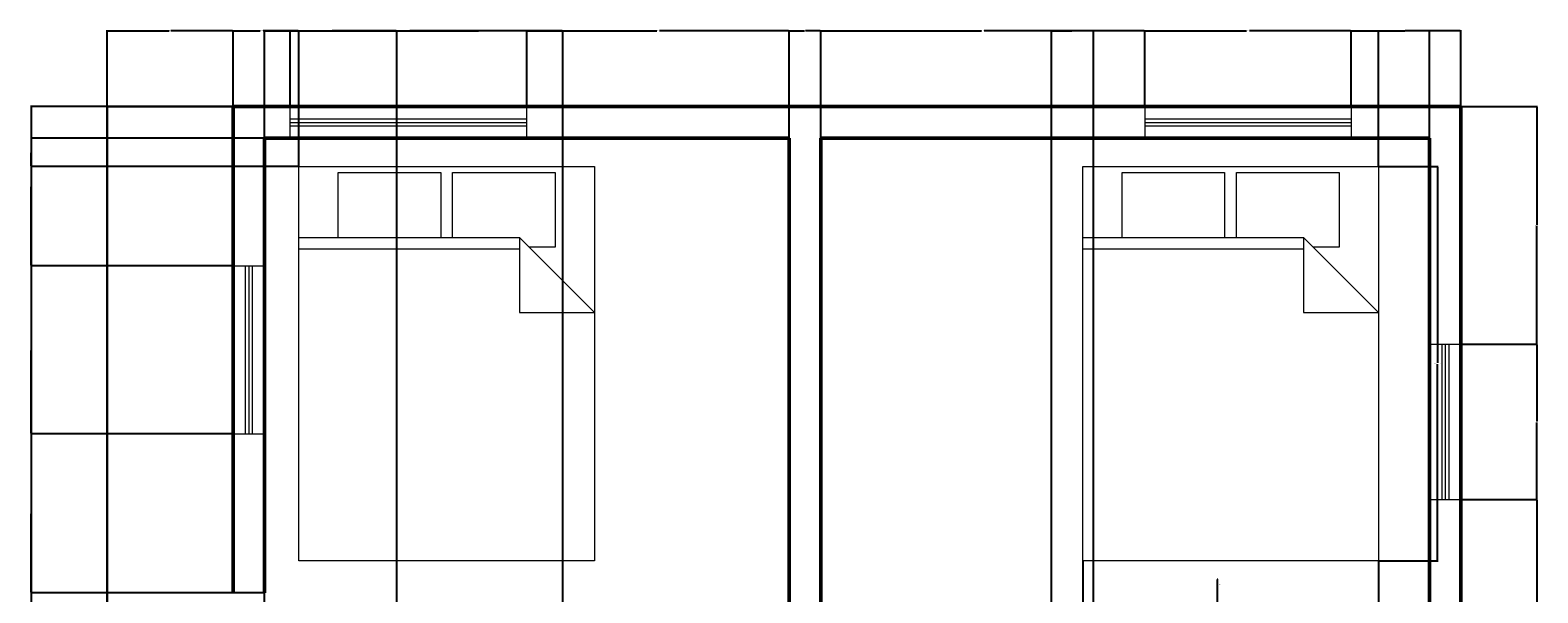
# Model space of a CAD drawing. Units: feet. Extents: x 2387 to 2818, y 1569 to 2046.
# Tile 4 of 4: x 2387 to 2818, y 1885 to 2046. Entities that reach past the tile are written whole.
import ezdxf

# ---------------------------------------------------------------- set-up
doc = ezdxf.new("R2010")
doc.units = ezdxf.units.FT
for name, color, linetype, lineweight in [('A-ANNO-DIMS', 2, 'Continuous', 18), ('A-DOOR', 3, 'Continuous', 25), ('A-FLOR-BALC', 7, 'Continuous', 30), ('A-FURN', 8, 'Continuous', 18), ('A-GLAZ', 4, 'Continuous', 18), ('A-WALL', 7, 'Continuous', 50)]:
    doc.layers.add(name, color=color, linetype=linetype, lineweight=lineweight)
doc.styles.get("Standard").update_dxf_attribs({"font": 'arial.ttf'})
doc.dimstyles.get("Standard").update_dxf_attribs({"dimtxt": 0.18, "dimasz": 0.18, "dimexe": 0.18, "dimexo": 0.0625, "dimgap": 0.09, "dimtad": 0, "dimtih": 1, "dimtoh": 1, "dimdec": 4, "dimzin": 0, "dimdsep": 46, "dimtxsty": 'Standard', "dimcen": 0.09, "dimadec": 0, "dimazin": 0, "dimtfac": 1, "dimtdec": 4, "dimtofl": 0, "dimtmove": 0, "dimatfit": 3, "dimfxl": 1, "dimtolj": 1, "dimtzin": 0, "dimarcsym": 0})

# ---------------------------------------------------------------- blocks, each defined once
blk = doc.blocks.new('Bed - Queen')
for p, q in [((0, -80.00003), (0, 0)), ((0, 0), (59.99999, 0)), ((59.99999, 0), (59.99999, -80.00003)), ((7.99999, -1.2), (28.79998, -1.2)), ((7.99999, -14.4), (7.99999, -1.2)), ((28.79998, -1.2), (28.79998, -14.4)), ((31.19999, -1.2), (51.99999, -1.2)), ((31.19999, -14.4), (31.19999, -1.2)), ((51.99999, -1.2), (51.99999, -16.4)), ((0, -14.4), (44.8, -14.4)), ((59.99999, -29.6), (44.8, -14.4)), ((44.8, -14.4), (44.8, -29.6)), ((44.8, -16.8), (0, -16.8)), ((51.99999, -16.4), (46.79936, -16.4)), ((44.8, -29.6), (59.99999, -29.6)), ((59.99999, -80.00003), (0, -80.00003))]:
    blk.add_line(p, q)
blk = doc.blocks.new('*D11')
at = {"layer": 'A-ANNO-DIMS', "color": 0, "lineweight": -2, "transparency": 16777216}
for p, q in [((2772.22, 2006.71), (2789.25, 2006.71)), ((2789.07, 2006.53), (2789.07, 1950.54)), ((2789.07, 1894.17), (2789.07, 1950.16)), ((2772.22, 1893.99), (2789.25, 1893.99))]:
    blk.add_line(p, q, dxfattribs=at)
at = {"layer": 'A-ANNO-DIMS', "color": 0, "transparency": 16777216}
for points in [[(2789.04, 2006.53), (2789.1, 2006.53), (2789.07, 2006.71)], [(2789.04, 1894.17), (2789.1, 1894.17), (2789.07, 1893.99)]]:
    blk.add_solid(points, dxfattribs=at)
at = {"layer": 'Defpoints', "color": 0, "transparency": 16777216}
for p in [(2772.16, 2006.71), (2789.07, 2006.71), (2772.16, 1893.99)]:
    blk.add_point(p, dxfattribs=at)
at = {"layer": 'A-ANNO-DIMS', "color": 0, "transparency": 16777216, "insert": (2789.07, 1950.35), "char_height": 0.18, "attachment_point": 5}
blk.add_mtext('\\A1;QUEEN BED 113 TYP.', dxfattribs=at)
blk = doc.blocks.new('*D12')
at = {"layer": 'A-ANNO-DIMS', "color": 0, "lineweight": -2, "transparency": 16777216}
for p, q in [((2687.62, 1893.93), (2687.62, 1876.9)), ((2772.16, 1893.93), (2772.16, 1876.9)), ((2687.8, 1877.08), (2729.36, 1877.08)), ((2771.98, 1877.08), (2730.42, 1877.08))]:
    blk.add_line(p, q, dxfattribs=at)
at = {"layer": 'A-ANNO-DIMS', "color": 0, "transparency": 16777216}
for points in [[(2687.8, 1877.11), (2687.8, 1877.05), (2687.62, 1877.08)], [(2771.98, 1877.11), (2771.98, 1877.05), (2772.16, 1877.08)]]:
    blk.add_solid(points, dxfattribs=at)
at = {"layer": 'Defpoints', "color": 0, "transparency": 16777216}
for p in [(2687.62, 1893.99), (2772.16, 1893.99), (2772.16, 1877.08)]:
    blk.add_point(p, dxfattribs=at)
at = {"layer": 'A-ANNO-DIMS', "color": 0, "transparency": 16777216, "insert": (2729.89, 1877.08), "char_height": 0.18, "attachment_point": 5}
blk.add_mtext('\\A1;85 TYP.', dxfattribs=at)
blk = doc.blocks.new('*D28')
at = {"layer": 'A-ANNO-DIMS', "color": 0, "lineweight": -2, "transparency": 16777216}
for p, q in [((2408.67, 2023.82), (2386.88, 2023.82)), ((2387.06, 2023.64), (2387.06, 1807.51)), ((2387.06, 1591), (2387.06, 1807.14)), ((2408.67, 1590.82), (2386.88, 1590.82))]:
    blk.add_line(p, q, dxfattribs=at)
at = {"layer": 'A-ANNO-DIMS', "color": 0, "transparency": 16777216}
for points in [[(2387.03, 2023.64), (2387.09, 2023.64), (2387.06, 2023.82)], [(2387.03, 1591), (2387.09, 1591), (2387.06, 1590.82)]]:
    blk.add_solid(points, dxfattribs=at)
at = {"layer": 'Defpoints', "color": 0, "transparency": 16777216}
for p in [(2387.06, 2023.82), (2408.74, 2023.82), (2408.74, 1590.82)]:
    blk.add_point(p, dxfattribs=at)
at = {"layer": 'A-ANNO-DIMS', "color": 0, "transparency": 16777216, "insert": (2387.06, 1807.32), "char_height": 0.18, "attachment_point": 5}
blk.add_mtext('\\A1;433', dxfattribs=at)
blk = doc.blocks.new('*D29')
at = {"layer": 'A-ANNO-DIMS', "color": 0, "lineweight": -2, "transparency": 16777216}
for p, q in [((2408.74, 2023.89), (2408.74, 2045.68)), ((2408.92, 2045.5), (2426.52, 2045.5)), ((2444.56, 2045.5), (2426.95, 2045.5)), ((2444.74, 2023.89), (2444.74, 2045.68))]:
    blk.add_line(p, q, dxfattribs=at)
at = {"layer": 'A-ANNO-DIMS', "color": 0, "transparency": 16777216}
for points in [[(2408.92, 2045.53), (2408.92, 2045.47), (2408.74, 2045.5)], [(2444.56, 2045.53), (2444.56, 2045.47), (2444.74, 2045.5)]]:
    blk.add_solid(points, dxfattribs=at)
at = {"layer": 'Defpoints', "color": 0, "transparency": 16777216}
for p in [(2444.74, 2045.5), (2408.74, 2023.82), (2444.74, 2023.82)]:
    blk.add_point(p, dxfattribs=at)
at = {"layer": 'A-ANNO-DIMS', "color": 0, "transparency": 16777216, "insert": (2426.74, 2045.5), "char_height": 0.18, "attachment_point": 5}
blk.add_mtext('\\A1;36', dxfattribs=at)
blk = doc.blocks.new('*D30')
at = {"layer": 'A-ANNO-DIMS', "color": 0, "lineweight": -2, "transparency": 16777216}
for p, q in [((2444.74, 2023.89), (2444.74, 2045.68)), ((2444.92, 2045.5), (2452.46, 2045.5)), ((2460.91, 2045.5), (2453.37, 2045.5)), ((2461.09, 2023.89), (2461.09, 2045.68))]:
    blk.add_line(p, q, dxfattribs=at)
at = {"layer": 'A-ANNO-DIMS', "color": 0, "transparency": 16777216}
for points in [[(2444.92, 2045.53), (2444.92, 2045.47), (2444.74, 2045.5)], [(2460.91, 2045.53), (2460.91, 2045.47), (2461.09, 2045.5)]]:
    blk.add_solid(points, dxfattribs=at)
at = {"layer": 'Defpoints', "color": 0, "transparency": 16777216}
for p in [(2461.09, 2045.5), (2444.74, 2023.82), (2461.09, 2023.82)]:
    blk.add_point(p, dxfattribs=at)
at = {"layer": 'A-ANNO-DIMS', "color": 0, "transparency": 16777216, "insert": (2452.91, 2045.5), "char_height": 0.18, "attachment_point": 5}
blk.add_mtext('\\A1;16.356', dxfattribs=at)
blk = doc.blocks.new('*D31')
at = {"layer": 'A-ANNO-DIMS', "color": 0, "lineweight": -2, "transparency": 16777216}
for p, q in [((2461.09, 2023.89), (2461.09, 2045.68)), ((2461.27, 2045.5), (2494.51, 2045.5)), ((2528.54, 2045.5), (2495.3, 2045.5)), ((2528.72, 2023.89), (2528.72, 2045.68))]:
    blk.add_line(p, q, dxfattribs=at)
at = {"layer": 'A-ANNO-DIMS', "color": 0, "transparency": 16777216}
for points in [[(2461.27, 2045.53), (2461.27, 2045.47), (2461.09, 2045.5)], [(2528.54, 2045.53), (2528.54, 2045.47), (2528.72, 2045.5)]]:
    blk.add_solid(points, dxfattribs=at)
at = {"layer": 'Defpoints', "color": 0, "transparency": 16777216}
for p in [(2528.72, 2045.5), (2461.09, 2023.82), (2528.72, 2023.82)]:
    blk.add_point(p, dxfattribs=at)
at = {"layer": 'A-ANNO-DIMS', "color": 0, "transparency": 16777216, "insert": (2494.91, 2045.5), "char_height": 0.18, "attachment_point": 5}
blk.add_mtext('\\A1;67.63', dxfattribs=at)
blk = doc.blocks.new('*D32')
at = {"layer": 'A-ANNO-DIMS', "color": 0, "lineweight": -2, "transparency": 16777216}
for p, q in [((2528.72, 2023.89), (2528.72, 2045.68)), ((2528.9, 2045.5), (2565.84, 2045.5)), ((2603.56, 2045.5), (2566.62, 2045.5)), ((2603.74, 2014.89), (2603.74, 2045.68))]:
    blk.add_line(p, q, dxfattribs=at)
at = {"layer": 'A-ANNO-DIMS', "color": 0, "transparency": 16777216}
for points in [[(2528.9, 2045.53), (2528.9, 2045.47), (2528.72, 2045.5)], [(2603.56, 2045.53), (2603.56, 2045.47), (2603.74, 2045.5)]]:
    blk.add_solid(points, dxfattribs=at)
at = {"layer": 'Defpoints', "color": 0, "transparency": 16777216}
for p in [(2603.74, 2045.5), (2528.72, 2023.82), (2603.74, 2014.82)]:
    blk.add_point(p, dxfattribs=at)
at = {"layer": 'A-ANNO-DIMS', "color": 0, "transparency": 16777216, "insert": (2566.23, 2045.5), "char_height": 0.18, "attachment_point": 5}
blk.add_mtext('\\A1;75.02', dxfattribs=at)
blk = doc.blocks.new('*D33')
at = {"layer": 'A-ANNO-DIMS', "color": 0, "lineweight": -2, "transparency": 16777216}
for p, q in [((2603.74, 2014.89), (2603.74, 2045.68)), ((2603.92, 2045.5), (2608.09, 2045.5)), ((2612.56, 2045.5), (2608.39, 2045.5)), ((2612.74, 2014.89), (2612.74, 2045.68))]:
    blk.add_line(p, q, dxfattribs=at)
at = {"layer": 'A-ANNO-DIMS', "color": 0, "transparency": 16777216}
for points in [[(2603.92, 2045.53), (2603.92, 2045.47), (2603.74, 2045.5)], [(2612.56, 2045.53), (2612.56, 2045.47), (2612.74, 2045.5)]]:
    blk.add_solid(points, dxfattribs=at)
at = {"layer": 'Defpoints', "color": 0, "transparency": 16777216}
for p in [(2612.74, 2045.5), (2603.74, 2014.82), (2612.74, 2014.82)]:
    blk.add_point(p, dxfattribs=at)
at = {"layer": 'A-ANNO-DIMS', "color": 0, "transparency": 16777216, "insert": (2608.24, 2045.5), "char_height": 0.18, "attachment_point": 5}
blk.add_mtext('\\A1;9', dxfattribs=at)
blk = doc.blocks.new('*D34')
at = {"layer": 'A-ANNO-DIMS', "color": 0, "lineweight": -2, "transparency": 16777216}
for p, q in [((2612.74, 2014.89), (2612.74, 2045.68)), ((2612.92, 2045.5), (2658.66, 2045.5)), ((2705.18, 2045.5), (2659.44, 2045.5)), ((2705.36, 2023.89), (2705.36, 2045.68))]:
    blk.add_line(p, q, dxfattribs=at)
at = {"layer": 'A-ANNO-DIMS', "color": 0, "transparency": 16777216}
for points in [[(2612.92, 2045.53), (2612.92, 2045.47), (2612.74, 2045.5)], [(2705.18, 2045.53), (2705.18, 2045.47), (2705.36, 2045.5)]]:
    blk.add_solid(points, dxfattribs=at)
at = {"layer": 'Defpoints', "color": 0, "transparency": 16777216}
for p in [(2705.36, 2045.5), (2705.36, 2023.82), (2612.74, 2014.82)]:
    blk.add_point(p, dxfattribs=at)
at = {"layer": 'A-ANNO-DIMS', "color": 0, "transparency": 16777216, "insert": (2659.05, 2045.5), "char_height": 0.18, "attachment_point": 5}
blk.add_mtext('\\A1;92.63', dxfattribs=at)
blk = doc.blocks.new('*D35')
at = {"layer": 'A-ANNO-DIMS', "color": 0, "lineweight": -2, "transparency": 16777216}
for p, q in [((2705.36, 2023.89), (2705.36, 2045.68)), ((2705.54, 2045.5), (2734.48, 2045.5)), ((2764.21, 2045.5), (2735.27, 2045.5)), ((2764.39, 2023.89), (2764.39, 2045.68))]:
    blk.add_line(p, q, dxfattribs=at)
at = {"layer": 'A-ANNO-DIMS', "color": 0, "transparency": 16777216}
for points in [[(2705.54, 2045.53), (2705.54, 2045.47), (2705.36, 2045.5)], [(2764.21, 2045.53), (2764.21, 2045.47), (2764.39, 2045.5)]]:
    blk.add_solid(points, dxfattribs=at)
at = {"layer": 'Defpoints', "color": 0, "transparency": 16777216}
for p in [(2764.39, 2045.5), (2705.36, 2023.82), (2764.39, 2023.82)]:
    blk.add_point(p, dxfattribs=at)
at = {"layer": 'A-ANNO-DIMS', "color": 0, "transparency": 16777216, "insert": (2734.88, 2045.5), "char_height": 0.18, "attachment_point": 5}
blk.add_mtext('\\A1;59.03', dxfattribs=at)
blk = doc.blocks.new('*D36')
at = {"layer": 'A-ANNO-DIMS', "color": 0, "lineweight": -2, "transparency": 16777216}
for p, q in [((2764.39, 2023.89), (2764.39, 2045.68)), ((2764.57, 2045.5), (2779.67, 2045.5)), ((2795.56, 2045.5), (2780.46, 2045.5)), ((2795.74, 2023.89), (2795.74, 2045.68))]:
    blk.add_line(p, q, dxfattribs=at)
at = {"layer": 'A-ANNO-DIMS', "color": 0, "transparency": 16777216}
for points in [[(2764.57, 2045.53), (2764.57, 2045.47), (2764.39, 2045.5)], [(2795.56, 2045.53), (2795.56, 2045.47), (2795.74, 2045.5)]]:
    blk.add_solid(points, dxfattribs=at)
at = {"layer": 'Defpoints', "color": 0, "transparency": 16777216}
for p in [(2795.74, 2045.5), (2764.39, 2023.82), (2795.74, 2023.82)]:
    blk.add_point(p, dxfattribs=at)
at = {"layer": 'A-ANNO-DIMS', "color": 0, "transparency": 16777216, "insert": (2780.07, 2045.5), "char_height": 0.18, "attachment_point": 5}
blk.add_mtext('\\A1;31.34', dxfattribs=at)
blk = doc.blocks.new('*D37')
at = {"layer": 'A-ANNO-DIMS', "color": 0, "lineweight": -2, "transparency": 16777216}
for p, q in [((2491.59, 1599.89), (2491.59, 2045.68)), ((2491.77, 2045.5), (2514.91, 2045.5)), ((2538.86, 2045.5), (2515.71, 2045.5)), ((2539.04, 1599.89), (2539.04, 2045.68))]:
    blk.add_line(p, q, dxfattribs=at)
at = {"layer": 'A-ANNO-DIMS', "color": 0, "transparency": 16777216}
for points in [[(2491.77, 2045.53), (2491.77, 2045.47), (2491.59, 2045.5)], [(2538.86, 2045.53), (2538.86, 2045.47), (2539.04, 2045.5)]]:
    blk.add_solid(points, dxfattribs=at)
at = {"layer": 'Defpoints', "color": 0, "transparency": 16777216}
for p in [(2539.04, 2045.5), (2491.59, 1599.82), (2539.04, 1599.82)]:
    blk.add_point(p, dxfattribs=at)
at = {"layer": 'A-ANNO-DIMS', "color": 0, "transparency": 16777216, "insert": (2515.31, 2045.5), "char_height": 0.18, "attachment_point": 5}
blk.add_mtext('\\A1;47.45', dxfattribs=at)
blk = doc.blocks.new('*D38')
at = {"layer": 'A-ANNO-DIMS', "color": 0, "lineweight": -2, "transparency": 16777216}
for p, q in [((2453.74, 1599.89), (2453.74, 2045.68)), ((2453.92, 2045.5), (2472.27, 2045.5)), ((2491.41, 2045.5), (2473.06, 2045.5)), ((2491.59, 1599.89), (2491.59, 2045.68))]:
    blk.add_line(p, q, dxfattribs=at)
at = {"layer": 'A-ANNO-DIMS', "color": 0, "transparency": 16777216}
for points in [[(2453.92, 2045.53), (2453.92, 2045.47), (2453.74, 2045.5)], [(2491.41, 2045.53), (2491.41, 2045.47), (2491.59, 2045.5)]]:
    blk.add_solid(points, dxfattribs=at)
at = {"layer": 'Defpoints', "color": 0, "transparency": 16777216}
for p in [(2491.59, 2045.5), (2453.74, 1599.82), (2491.59, 1599.82)]:
    blk.add_point(p, dxfattribs=at)
at = {"layer": 'A-ANNO-DIMS', "color": 0, "transparency": 16777216, "insert": (2472.66, 2045.5), "char_height": 0.18, "attachment_point": 5}
blk.add_mtext('\\A1;37.85', dxfattribs=at)
blk = doc.blocks.new('*D47')
at = {"layer": 'A-ANNO-DIMS', "color": 0, "lineweight": -2, "transparency": 16777216}
for p, q in [((2444.67, 1930.32), (2386.88, 1930.32)), ((2387.06, 1930.14), (2387.06, 1907.76)), ((2387.06, 1885), (2387.06, 1907.39)), ((2444.67, 1884.82), (2386.88, 1884.82))]:
    blk.add_line(p, q, dxfattribs=at)
at = {"layer": 'A-ANNO-DIMS', "color": 0, "transparency": 16777216}
for points in [[(2387.03, 1930.14), (2387.09, 1930.14), (2387.06, 1930.32)], [(2387.03, 1885), (2387.09, 1885), (2387.06, 1884.82)]]:
    blk.add_solid(points, dxfattribs=at)
at = {"layer": 'Defpoints', "color": 0, "transparency": 16777216}
for p in [(2387.06, 1930.32), (2444.74, 1930.32), (2444.74, 1884.82)]:
    blk.add_point(p, dxfattribs=at)
at = {"layer": 'A-ANNO-DIMS', "color": 0, "transparency": 16777216, "insert": (2387.06, 1907.57), "char_height": 0.18, "attachment_point": 5}
blk.add_mtext('\\A1;45.5', dxfattribs=at)
blk = doc.blocks.new('*D48')
at = {"layer": 'A-ANNO-DIMS', "color": 0, "lineweight": -2, "transparency": 16777216}
for p, q in [((2444.67, 1978.32), (2386.88, 1978.32)), ((2387.06, 1978.14), (2387.06, 1954.51)), ((2387.06, 1930.5), (2387.06, 1954.14)), ((2444.67, 1930.32), (2386.88, 1930.32))]:
    blk.add_line(p, q, dxfattribs=at)
at = {"layer": 'A-ANNO-DIMS', "color": 0, "transparency": 16777216}
for points in [[(2387.03, 1978.14), (2387.09, 1978.14), (2387.06, 1978.32)], [(2387.03, 1930.5), (2387.09, 1930.5), (2387.06, 1930.32)]]:
    blk.add_solid(points, dxfattribs=at)
at = {"layer": 'Defpoints', "color": 0, "transparency": 16777216}
for p in [(2387.06, 1978.32), (2444.74, 1978.32), (2444.74, 1930.32)]:
    blk.add_point(p, dxfattribs=at)
at = {"layer": 'A-ANNO-DIMS', "color": 0, "transparency": 16777216, "insert": (2387.06, 1954.32), "char_height": 0.18, "attachment_point": 5}
blk.add_mtext('\\A1;48', dxfattribs=at)
blk = doc.blocks.new('*D49')
at = {"layer": 'A-ANNO-DIMS', "color": 0, "lineweight": -2, "transparency": 16777216}
for p, q in [((2444.67, 2023.82), (2386.88, 2023.82)), ((2387.06, 2023.64), (2387.06, 2001.26)), ((2387.06, 1978.5), (2387.06, 2000.89)), ((2444.67, 1978.32), (2386.88, 1978.32))]:
    blk.add_line(p, q, dxfattribs=at)
at = {"layer": 'A-ANNO-DIMS', "color": 0, "transparency": 16777216}
for points in [[(2387.03, 2023.64), (2387.09, 2023.64), (2387.06, 2023.82)], [(2387.03, 1978.5), (2387.09, 1978.5), (2387.06, 1978.32)]]:
    blk.add_solid(points, dxfattribs=at)
at = {"layer": 'Defpoints', "color": 0, "transparency": 16777216}
for p in [(2387.06, 2023.82), (2444.74, 2023.82), (2444.74, 1978.32)]:
    blk.add_point(p, dxfattribs=at)
at = {"layer": 'A-ANNO-DIMS', "color": 0, "transparency": 16777216, "insert": (2387.06, 2001.07), "char_height": 0.18, "attachment_point": 5}
blk.add_mtext('\\A1;45.5', dxfattribs=at)
blk = doc.blocks.new('*D54')
at = {"layer": 'A-ANNO-DIMS', "color": 0, "lineweight": -2, "transparency": 16777216}
for p, q in [((2795.8, 1911.52), (2817.6, 1911.52)), ((2817.42, 1911.34), (2817.42, 1861.45)), ((2817.42, 1811.2), (2817.42, 1861.09)), ((2795.8, 1811.02), (2817.6, 1811.02))]:
    blk.add_line(p, q, dxfattribs=at)
at = {"layer": 'A-ANNO-DIMS', "color": 0, "transparency": 16777216}
for points in [[(2817.39, 1911.34), (2817.45, 1911.34), (2817.42, 1911.52)], [(2817.39, 1811.2), (2817.45, 1811.2), (2817.42, 1811.02)]]:
    blk.add_solid(points, dxfattribs=at)
at = {"layer": 'Defpoints', "color": 0, "transparency": 16777216}
for p in [(2795.74, 1911.52), (2817.42, 1911.52), (2795.74, 1811.02)]:
    blk.add_point(p, dxfattribs=at)
at = {"layer": 'A-ANNO-DIMS', "color": 0, "transparency": 16777216, "insert": (2817.42, 1861.27), "char_height": 0.18, "attachment_point": 5}
blk.add_mtext('\\A1;100.5', dxfattribs=at)
blk = doc.blocks.new('*D55')
at = {"layer": 'A-ANNO-DIMS', "color": 0, "lineweight": -2, "transparency": 16777216}
for p, q in [((2795.8, 1955.94), (2817.6, 1955.94)), ((2817.42, 1955.76), (2817.42, 1933.91)), ((2817.42, 1911.7), (2817.42, 1933.55)), ((2795.8, 1911.52), (2817.6, 1911.52))]:
    blk.add_line(p, q, dxfattribs=at)
at = {"layer": 'A-ANNO-DIMS', "color": 0, "transparency": 16777216}
for points in [[(2817.39, 1955.76), (2817.45, 1955.76), (2817.42, 1955.94)], [(2817.39, 1911.7), (2817.45, 1911.7), (2817.42, 1911.52)]]:
    blk.add_solid(points, dxfattribs=at)
at = {"layer": 'Defpoints', "color": 0, "transparency": 16777216}
for p in [(2795.74, 1955.94), (2817.42, 1955.94), (2795.74, 1911.52)]:
    blk.add_point(p, dxfattribs=at)
at = {"layer": 'A-ANNO-DIMS', "color": 0, "transparency": 16777216, "insert": (2817.42, 1933.73), "char_height": 0.18, "attachment_point": 5}
blk.add_mtext('\\A1;44.42', dxfattribs=at)
blk = doc.blocks.new('*D56')
at = {"layer": 'A-ANNO-DIMS', "color": 0, "lineweight": -2, "transparency": 16777216}
for p, q in [((2795.8, 2023.82), (2817.6, 2023.82)), ((2817.42, 2023.64), (2817.42, 1990.06)), ((2817.42, 1956.12), (2817.42, 1989.7)), ((2795.8, 1955.94), (2817.6, 1955.94))]:
    blk.add_line(p, q, dxfattribs=at)
at = {"layer": 'A-ANNO-DIMS', "color": 0, "transparency": 16777216}
for points in [[(2817.39, 2023.64), (2817.45, 2023.64), (2817.42, 2023.82)], [(2817.39, 1956.12), (2817.45, 1956.12), (2817.42, 1955.94)]]:
    blk.add_solid(points, dxfattribs=at)
at = {"layer": 'Defpoints', "color": 0, "transparency": 16777216}
for p in [(2795.74, 2023.82), (2817.42, 2023.82), (2795.74, 1955.94)]:
    blk.add_point(p, dxfattribs=at)
at = {"layer": 'A-ANNO-DIMS', "color": 0, "transparency": 16777216, "insert": (2817.42, 1989.88), "char_height": 0.18, "attachment_point": 5}
blk.add_mtext('\\A1;67.89', dxfattribs=at)
blk = doc.blocks.new('*D58')
at = {"layer": 'A-ANNO-DIMS', "color": 0, "lineweight": -2, "transparency": 16777216}
for p, q in [((2678.74, 1646.89), (2678.74, 2045.68)), ((2678.92, 2045.5), (2684.53, 2045.5)), ((2690.56, 2045.5), (2684.95, 2045.5)), ((2690.74, 1646.89), (2690.74, 2045.68))]:
    blk.add_line(p, q, dxfattribs=at)
at = {"layer": 'A-ANNO-DIMS', "color": 0, "transparency": 16777216}
for points in [[(2678.92, 2045.53), (2678.92, 2045.47), (2678.74, 2045.5)], [(2690.56, 2045.53), (2690.56, 2045.47), (2690.74, 2045.5)]]:
    blk.add_solid(points, dxfattribs=at)
at = {"layer": 'Defpoints', "color": 0, "transparency": 16777216}
for p in [(2690.74, 2045.5), (2678.74, 1646.82), (2690.74, 1646.82)]:
    blk.add_point(p, dxfattribs=at)
at = {"layer": 'A-ANNO-DIMS', "color": 0, "transparency": 16777216, "insert": (2684.74, 2045.5), "char_height": 0.18, "attachment_point": 5}
blk.add_mtext('\\A1;12', dxfattribs=at)
blk = doc.blocks.new('*D64')
at = {"layer": 'A-ANNO-DIMS', "color": 0, "lineweight": -2, "transparency": 16777216}
for p, q in [((2453.74, 2014.89), (2453.74, 2045.68)), ((2453.92, 2045.5), (2458.23, 2045.5)), ((2463.34, 2045.5), (2459.02, 2045.5)), ((2463.52, 2006.77), (2463.52, 2045.68))]:
    blk.add_line(p, q, dxfattribs=at)
at = {"layer": 'A-ANNO-DIMS', "color": 0, "transparency": 16777216}
for points in [[(2453.92, 2045.53), (2453.92, 2045.47), (2453.74, 2045.5)], [(2463.34, 2045.53), (2463.34, 2045.47), (2463.52, 2045.5)]]:
    blk.add_solid(points, dxfattribs=at)
at = {"layer": 'Defpoints', "color": 0, "transparency": 16777216}
for p in [(2453.74, 2045.5), (2453.74, 2014.82), (2463.52, 2006.71)]:
    blk.add_point(p, dxfattribs=at)
at = {"layer": 'A-ANNO-DIMS', "color": 0, "transparency": 16777216, "insert": (2458.63, 2045.5), "char_height": 0.18, "attachment_point": 5}
blk.add_mtext('\\A1;9.784', dxfattribs=at)
blk = doc.blocks.new('*D65')
at = {"layer": 'A-ANNO-DIMS', "color": 0, "lineweight": -2, "transparency": 16777216}
for p, q in [((2453.67, 2014.82), (2386.88, 2014.82)), ((2387.06, 2014.64), (2387.06, 2010.95)), ((2387.06, 2006.89), (2387.06, 2010.59)), ((2463.46, 2006.71), (2386.88, 2006.71))]:
    blk.add_line(p, q, dxfattribs=at)
at = {"layer": 'A-ANNO-DIMS', "color": 0, "transparency": 16777216}
for points in [[(2387.03, 2014.64), (2387.09, 2014.64), (2387.06, 2014.82)], [(2387.03, 2006.89), (2387.09, 2006.89), (2387.06, 2006.71)]]:
    blk.add_solid(points, dxfattribs=at)
at = {"layer": 'Defpoints', "color": 0, "transparency": 16777216}
for p in [(2387.06, 2014.82), (2453.74, 2014.82), (2463.52, 2006.71)]:
    blk.add_point(p, dxfattribs=at)
at = {"layer": 'A-ANNO-DIMS', "color": 0, "transparency": 16777216, "insert": (2387.06, 2010.77), "char_height": 0.18, "attachment_point": 5}
blk.add_mtext('\\A1;8.113', dxfattribs=at)
blk = doc.blocks.new('*D66')
at = {"layer": 'A-ANNO-DIMS', "color": 0, "lineweight": -2, "transparency": 16777216}
for p, q in [((2772.16, 2006.77), (2772.16, 2045.68)), ((2772.34, 2045.5), (2779.06, 2045.5)), ((2786.56, 2045.5), (2779.83, 2045.5)), ((2786.74, 2014.89), (2786.74, 2045.68))]:
    blk.add_line(p, q, dxfattribs=at)
at = {"layer": 'A-ANNO-DIMS', "color": 0, "transparency": 16777216}
for points in [[(2772.34, 2045.53), (2772.34, 2045.47), (2772.16, 2045.5)], [(2786.56, 2045.53), (2786.56, 2045.47), (2786.74, 2045.5)]]:
    blk.add_solid(points, dxfattribs=at)
at = {"layer": 'Defpoints', "color": 0, "transparency": 16777216}
for p in [(2786.74, 2045.5), (2786.74, 2014.82), (2772.16, 2006.71)]:
    blk.add_point(p, dxfattribs=at)
at = {"layer": 'A-ANNO-DIMS', "color": 0, "transparency": 16777216, "insert": (2779.45, 2045.5), "char_height": 0.18, "attachment_point": 5}
blk.add_mtext('\\A1;14.58', dxfattribs=at)
blk = doc.blocks.new('*D76')
at = {"layer": 'A-ANNO-DIMS', "color": 0, "lineweight": -2, "transparency": 16777216}
for p, q in [((2726.29, 1887.29), (2726.1, 1887.29)), ((2726.1, 1887.29), (2726.1, 1833.83)), ((2726.01, 1744.25), (2726.19, 1744.25)), ((2726.1, 1744.16), (2726.1, 1744.34))]:
    blk.add_line(p, q, dxfattribs=at)
at = {"layer": 'A-ANNO-DIMS', "color": 0, "transparency": 16777216}
blk.add_solid([(2726.08, 1833.83), (2726.14, 1833.83), (2726.1, 1833.65)], dxfattribs=at)
at = {"layer": 'Defpoints', "color": 0, "transparency": 16777216}
for p in [(2726.1, 1833.65), (2726.1, 1744.25)]:
    blk.add_point(p, dxfattribs=at)
at = {"layer": 'A-ANNO-DIMS', "color": 0, "transparency": 16777216, "insert": (2726.69, 1887.29), "char_height": 0.18, "attachment_point": 5}
blk.add_mtext('\\A1;R89.4', dxfattribs=at)
blk = doc.blocks.new('*D77')
at = {"layer": 'A-ANNO-DIMS', "color": 0, "lineweight": -2, "transparency": 16777216}
for p, q in [((2726.29, 1888.64), (2726.1, 1888.64)), ((2726.1, 1888.64), (2726.1, 1838.25)), ((2726.01, 1753.8), (2726.19, 1753.8)), ((2726.1, 1753.71), (2726.1, 1753.89))]:
    blk.add_line(p, q, dxfattribs=at)
at = {"layer": 'A-ANNO-DIMS', "color": 0, "transparency": 16777216}
blk.add_solid([(2726.08, 1838.25), (2726.14, 1838.25), (2726.1, 1838.07)], dxfattribs=at)
at = {"layer": 'Defpoints', "color": 0, "transparency": 16777216}
for p in [(2726.1, 1838.07), (2726.1, 1753.8)]:
    blk.add_point(p, dxfattribs=at)
at = {"layer": 'A-ANNO-DIMS', "color": 0, "transparency": 16777216, "insert": (2726.76, 1888.64), "char_height": 0.18, "attachment_point": 5}
blk.add_mtext('\\A1;R84.27', dxfattribs=at)

msp = doc.modelspace()

# ---------------------------------------------------------------- linework, layer by layer
at = {"layer": 'A-DOOR'}
msp.add_line((2453.736, 1884.8244), (2444.736, 1884.8244), dxfattribs=at)
at = {"layer": 'A-FLOR-BALC'}
for p, q in [((2444.736, 2023.8244), (2408.736, 2023.8244)), ((2408.736, 2023.8244), (2408.736, 1590.8244))]:
    msp.add_line(p, q, dxfattribs=at)
at = {"layer": 'A-GLAZ'}
for p, q in [((2461.0918, 2014.8244), (2461.0918, 2023.8244)), ((2528.7185, 2014.8244), (2528.7185, 2023.8244)), ((2705.3619, 2023.8244), (2705.3619, 2014.8244)), ((2764.3946, 2023.8244), (2764.3946, 2014.8244)), ((2461.0918, 2020.3244), (2528.7185, 2020.3244)), ((2461.0918, 2019.3244), (2528.7185, 2019.3244)), ((2461.0918, 2018.3244), (2528.7185, 2018.3244)), ((2705.3619, 2020.3244), (2764.3946, 2020.3244)), ((2705.3619, 2019.3244), (2764.3946, 2019.3244)), ((2705.3619, 2018.3244), (2764.3946, 2018.3244)), ((2444.736, 1978.3244), (2453.736, 1978.3244)), ((2448.236, 1978.3244), (2448.236, 1930.3244)), ((2449.236, 1978.3244), (2449.236, 1930.3244)), ((2450.236, 1978.3244), (2450.236, 1930.3244)), ((2786.736, 1955.9362), (2795.736, 1955.9362)), ((2790.236, 1955.9362), (2790.236, 1911.5166)), ((2791.236, 1955.9362), (2791.236, 1911.5166)), ((2792.236, 1955.9362), (2792.236, 1911.5166)), ((2444.736, 1930.3244), (2453.736, 1930.3244)), ((2786.736, 1911.5166), (2795.736, 1911.5166))]:
    msp.add_line(p, q, dxfattribs=at)
at = {"layer": 'A-WALL'}
for p, q in [((2444.736, 2023.8244), (2795.736, 2023.8244)), ((2444.736, 1884.8244), (2444.736, 2023.8244)), ((2612.736, 2023.8244), (2795.736, 2023.8244)), ((2795.736, 2023.8244), (2795.736, 1722.8244)), ((2453.736, 2014.8244), (2603.736, 2014.8244)), ((2453.736, 1884.8244), (2453.736, 2014.8244)), ((2603.736, 2014.8244), (2603.736, 1839.8244)), ((2612.736, 2014.8244), (2612.736, 1839.8244)), ((2612.736, 2014.8244), (2786.736, 2014.8244)), ((2786.736, 2014.8244), (2786.736, 1848.8244)), ((2444.736, 1954.3244), (2444.736, 1924.6386))]:
    msp.add_line(p, q, dxfattribs=at)

# ---------------------------------------------------------------- block references
at = {"layer": 'A-FURN', "xscale": 1.409007892519721, "yscale": 1.409007892519721, "zscale": 1.409007892519721}
for p in [(2463.5203, 2006.7119), (2687.6167, 2006.7119)]:
    msp.add_blockref('Bed - Queen', p, dxfattribs=at)

# ---------------------------------------------------------------- dimensions: what is measured, and where the dimension line sits
at = {"layer": 'A-ANNO-DIMS'}
for base, p1, p2, override, picture, middle in [((2444.736, 2045.5044), (2408.736, 2023.8244), (2444.736, 2023.8244), {"dimdec": 0, "dimlfac": 1, "dimrnd": 0, "dimzin": 0, "dimdsep": 46, "dimlunit": 2}, '*D29', (2426.736, 2045.5044)), ((2461.0918, 2045.5044), (2444.736, 2023.8244), (2461.0918, 2023.8244), {"dimdec": 3, "dimlfac": 1, "dimrnd": 0, "dimzin": 0, "dimdsep": 46, "dimlunit": 2}, '*D30', (2452.9139, 2045.5044)), ((2491.5876, 2045.5044), (2453.736, 1599.8244), (2491.5876, 1599.8244), {"dimdec": 2, "dimlfac": 1, "dimrnd": 0, "dimzin": 0, "dimdsep": 46, "dimlunit": 2}, '*D38', (2472.6618, 2045.5044)), ((2453.736, 2045.5044), (2463.5203, 2006.7119), (2453.736, 2014.8244), {"dimdec": 3, "dimlfac": 1, "dimrnd": 0, "dimzin": 0, "dimdsep": 46, "dimlunit": 2}, '*D64', (2458.6281, 2045.5044)), ((2528.7185, 2045.5044), (2461.0918, 2023.8244), (2528.7185, 2023.8244), {"dimdec": 2, "dimlfac": 1, "dimrnd": 0, "dimzin": 0, "dimdsep": 46, "dimlunit": 2}, '*D31', (2494.9052, 2045.5044)), ((2539.0379, 2045.5044), (2491.5876, 1599.8244), (2539.0379, 1599.8244), {"dimdec": 2, "dimlfac": 1, "dimrnd": 0, "dimzin": 0, "dimdsep": 46, "dimlunit": 2}, '*D37', (2515.3128, 2045.5044)), ((2603.736, 2045.5044), (2528.7185, 2023.8244), (2603.736, 2014.8244), {"dimdec": 2, "dimlfac": 1, "dimrnd": 0, "dimzin": 0, "dimdsep": 46, "dimlunit": 2}, '*D32', (2566.2272, 2045.5044)), ((2612.736, 2045.5044), (2603.736, 2014.8244), (2612.736, 2014.8244), {"dimdec": 0, "dimlfac": 1, "dimrnd": 0, "dimzin": 0, "dimdsep": 46, "dimlunit": 2}, '*D33', (2608.236, 2045.5044)), ((2705.3619, 2045.5044), (2612.736, 2014.8244), (2705.3619, 2023.8244), {"dimdec": 2, "dimlfac": 1, "dimrnd": 0, "dimzin": 0, "dimdsep": 46, "dimlunit": 2}, '*D34', (2659.0489, 2045.5044)), ((2690.736, 2045.5044), (2678.736, 1646.8244), (2690.736, 1646.8244), {"dimdec": 0, "dimlfac": 1, "dimrnd": 0, "dimzin": 0, "dimdsep": 46, "dimlunit": 2}, '*D58', (2684.736, 2045.5044)), ((2764.3946, 2045.5044), (2705.3619, 2023.8244), (2764.3946, 2023.8244), {"dimdec": 2, "dimlfac": 1, "dimrnd": 0, "dimzin": 0, "dimdsep": 46, "dimlunit": 2}, '*D35', (2734.8783, 2045.5044)), ((2795.736, 2045.5044), (2764.3946, 2023.8244), (2795.736, 2023.8244), {"dimdec": 2, "dimlfac": 1, "dimrnd": 0, "dimzin": 0, "dimdsep": 46, "dimlunit": 2}, '*D36', (2780.0653, 2045.5044)), ((2786.736, 2045.5044), (2772.1572, 2006.7119), (2786.736, 2014.8244), {"dimdec": 2, "dimlfac": 1, "dimrnd": 0, "dimzin": 0, "dimdsep": 46, "dimlunit": 2}, '*D66', (2779.4466, 2045.5044))]:
    dim = msp.add_linear_dim(base=base, p1=p1, p2=p2, dimstyle='Standard', override=override, dxfattribs=at)
    dim.commit()
    dim.dimension.update_dxf_attribs({"geometry": picture, "text_midpoint": middle})
for base, p1, p2, override, picture, middle in [((2387.056, 2023.8244), (2444.736, 1978.3244), (2444.736, 2023.8244), {"dimdec": 1, "dimlfac": 1, "dimrnd": 0, "dimzin": 0, "dimdsep": 46, "dimlunit": 2}, '*D49', (2387.056, 2001.0744)), ((2387.056, 2023.8244), (2408.736, 1590.8244), (2408.736, 2023.8244), {"dimdec": 0, "dimlfac": 1, "dimrnd": 0, "dimzin": 0, "dimdsep": 46, "dimlunit": 2}, '*D28', (2387.056, 1807.3244)), ((2817.416, 2023.8244), (2795.736, 1955.9362), (2795.736, 2023.8244), {"dimdec": 2, "dimlfac": 1, "dimrnd": 0, "dimzin": 0, "dimdsep": 46, "dimlunit": 2}, '*D56', (2817.416, 1989.8803)), ((2387.05596, 2014.82441), (2463.52027, 2006.71187), (2453.73596, 2014.82441), {"dimdec": 3, "dimlfac": 1, "dimrnd": 0, "dimzin": 0, "dimdsep": 46, "dimlunit": 2}, '*D65', (2387.05596, 2010.76814)), ((2387.056, 1978.3244), (2444.736, 1930.3244), (2444.736, 1978.3244), {"dimdec": 0, "dimlfac": 1, "dimrnd": 0, "dimzin": 0, "dimdsep": 46, "dimlunit": 2}, '*D48', (2387.056, 1954.3244)), ((2817.416, 1955.9362), (2795.736, 1911.5166), (2795.736, 1955.9362), {"dimdec": 2, "dimlfac": 1, "dimrnd": 0, "dimzin": 0, "dimdsep": 46, "dimlunit": 2}, '*D55', (2817.416, 1933.7264)), ((2387.056, 1930.3244), (2444.736, 1884.8244), (2444.736, 1930.3244), {"dimdec": 1, "dimlfac": 1, "dimrnd": 0, "dimzin": 0, "dimdsep": 46, "dimlunit": 2}, '*D47', (2387.056, 1907.5744)), ((2817.416, 1911.5166), (2795.736, 1811.0226), (2795.736, 1911.5166), {"dimdec": 1, "dimlfac": 1, "dimrnd": 0, "dimzin": 0, "dimdsep": 46, "dimlunit": 2}, '*D54', (2817.416, 1861.2696))]:
    dim = msp.add_linear_dim(base=base, p1=p1, p2=p2, angle=90, dimstyle='Standard', override=override, dxfattribs=at)
    dim.commit()
    dim.dimension.update_dxf_attribs({"geometry": picture, "text_midpoint": middle})
dim = msp.add_linear_dim(base=(2789.0653, 2006.7119), p1=(2772.1572, 1893.9912), p2=(2772.1572, 2006.7119), angle=90, text='QUEEN BED <> TYP.', dimstyle='Standard', override={"dimdec": 0, "dimlfac": 1, "dimrnd": 0, "dimzin": 0, "dimdsep": 46, "dimlunit": 2}, dxfattribs=at)
dim.commit()
dim.dimension.update_dxf_attribs({"geometry": '*D11', "text_midpoint": (2789.0653, 1950.3515)})
dim = msp.add_linear_dim(base=(2772.1572, 1877.0831), p1=(2687.6167, 1893.9912), p2=(2772.1572, 1893.9912), text='<> TYP.', dimstyle='Standard', override={"dimdec": 0, "dimlfac": 1, "dimrnd": 0, "dimzin": 0, "dimdsep": 46, "dimlunit": 2}, dxfattribs=at)
dim.commit()
dim.dimension.update_dxf_attribs({"geometry": '*D12', "text_midpoint": (2729.887, 1877.0831)})
for center, mpoint, override, picture, middle in [((2726.1049, 1753.7998), (2726.105, 1838.0742), {"dimdec": 2, "dimlfac": 1, "dimrnd": 0, "dimzin": 0, "dimdsep": 46, "dimlunit": 2}, '*D77', (2726.7649, 1888.6388)), ((2726.1049, 1744.2498), (2726.105, 1833.6484), {"dimdec": 1, "dimlfac": 1, "dimrnd": 0, "dimzin": 0, "dimdsep": 46, "dimlunit": 2}, '*D76', (2726.6946, 1887.2876))]:
    dim = msp.add_radius_dim(center=center, mpoint=mpoint, dimstyle='Standard', override=override, dxfattribs=at)
    dim.commit()
    dim.dimension.update_dxf_attribs({"geometry": picture, "text_midpoint": middle, "dimtype": 164})

doc.saveas('drawing.dxf')
